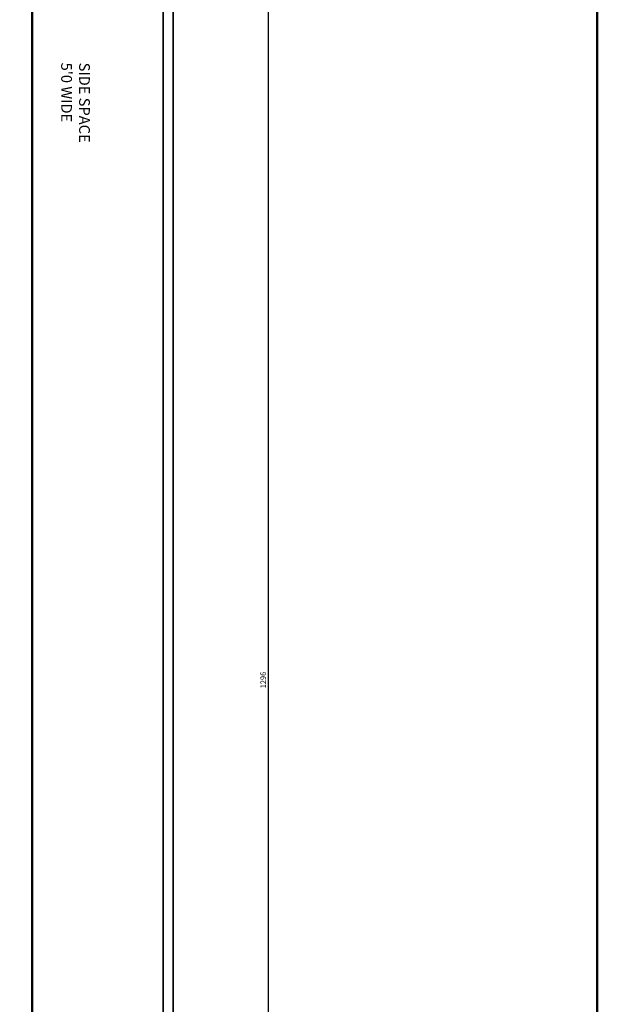
# Model space of a CAD drawing. Units: millimetres. Extents: x 2134 to 3363, y 1052 to 3233.
# Tile 8 of 11: x 3099 to 3363, y 2268 to 2718. Entities that reach past the tile are written whole.
import ezdxf

# ---------------------------------------------------------------- set-up
doc = ezdxf.new("R2010")
doc.units = ezdxf.units.MM
for name, color, linetype, lineweight in [('A-ANNO-DIMS', 2, 'Continuous', 18), ('A-ANNO-TTLB', 7, 'Continuous', 50), ('A-AREA-IDEN', 3, 'Continuous', 18), ('A-WALL', 7, 'Continuous', 50), ('C-PROP', 6, 'Continuous', 35)]:
    doc.layers.add(name, color=color, linetype=linetype, lineweight=lineweight)
doc.styles.get("Standard").update_dxf_attribs({"font": 'arial.ttf'})
doc.styles.add('YQ_DIM', font='SUPEROS.SHX', dxfattribs={"width": 0.8, "bigfont": 'HZDX.SHX'})
doc.dimstyles.new('ISO-25', dxfattribs={"dimtxt": 2.5, "dimasz": 2.5, "dimexe": 1.25, "dimexo": 0.625, "dimtad": 1, "dimtxsty": 'Standard', "dimcen": 2.5, "dimadec": 0, "dimazin": 0, "dimtfac": 1, "dimtmove": 0, "dimatfit": 3, "dimfxl": 1, "dimarcsym": 0})

# ---------------------------------------------------------------- blocks, each defined once
blk = doc.blocks.new('*D9')
at = {"layer": 'A-ANNO-DIMS', "color": 0, "lineweight": -2, "transparency": 16777216}
for p, q in [((3169.46, 3063.82), (3213.48, 3063.82)), ((3212.23, 3061.32), (3212.23, 1770.32)), ((3169.46, 1767.82), (3213.48, 1767.82))]:
    blk.add_line(p, q, dxfattribs=at)
at = {"layer": 'A-ANNO-DIMS', "color": 0, "transparency": 16777216}
for points in [[(3211.81, 3061.32), (3212.65, 3061.32), (3212.23, 3063.82)], [(3211.81, 1770.32), (3212.65, 1770.32), (3212.23, 1767.82)]]:
    blk.add_solid(points, dxfattribs=at)
at = {"layer": 'Defpoints', "color": 0, "transparency": 16777216}
for p in [(3168.84, 3063.82), (3168.84, 1767.82), (3212.23, 1767.82)]:
    blk.add_point(p, dxfattribs=at)
at = {"layer": 'A-ANNO-DIMS', "color": 0, "transparency": 16777216, "insert": (3210.33, 2415.82), "char_height": 2.5, "attachment_point": 5, "rotation": 90}
blk.add_mtext('1296', dxfattribs=at)

msp = doc.modelspace()

# ---------------------------------------------------------------- linework, layer by layer
at = {"layer": 'A-ANNO-TTLB', "ltscale": 0.5}
msp.add_lwpolyline([(2134.34, 3233.23), (3362.77, 3233.23), (3362.77, 1152.237), (2134.34, 1152.237)], close=True, dxfattribs=at)
at = {"layer": 'A-WALL'}
for q in [(3104.339, 2017.274), (3104.339, 2006.774)]:
    msp.add_line((3104.339, 3021.274), q, dxfattribs=at)
at = {"layer": 'C-PROP'}
for p, q in [((3168.839, 3063.82), (3168.839, 1767.82)), ((3164.339, 3059.32), (3164.339, 1770.366))]:
    msp.add_line(p, q, dxfattribs=at)

# ---------------------------------------------------------------- texts
at = {"layer": 'A-AREA-IDEN', "insert": (3130.772, 2697.896), "char_height": 4.91305, "attachment_point": 1, "rotation": 270, "style": 'YQ_DIM'}
msp.add_mtext_dynamic_manual_height_columns("{\\f@Arial Unicode MS|b0|i0|c134|p34;SIDE SPACE\\P5'0 WIDE}", width=92.43125, gutter_width=24.565, heights=[0], dxfattribs=at)

# ---------------------------------------------------------------- dimensions: what is measured, and where the dimension line sits
at = {"layer": 'A-ANNO-DIMS'}
dim = msp.add_linear_dim(base=(3212.229, 1767.82), p1=(3168.839, 3063.82), p2=(3168.839, 1767.82), angle=90, dimstyle='ISO-25', override={"dimclrd": 0, "dimclre": 0, "dimclrt": 0}, dxfattribs=at)
dim.commit()
dim.dimension.update_dxf_attribs({"geometry": '*D9', "text_midpoint": (3210.327, 2415.82)})

doc.saveas('drawing.dxf')
